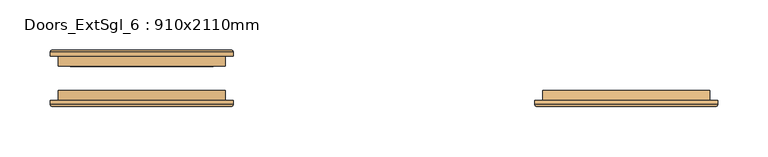
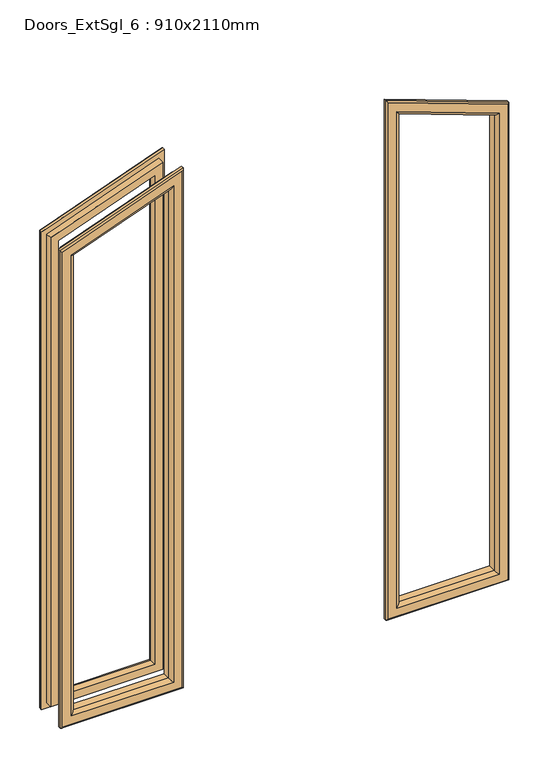
"""IFC4 building model written with IfcOpenShell, lengths in millimetres: door geometry, Doors_ExtSgl_6 : 910x2110mm."""

from ifc_helpers import new_model, si_unit, frame, origin, place, context, project, spatial, ellipse_curve, source, transform, mapped, element, save
from ifc_brep_helpers import plane_surface, cylinder_surface, advanced_brep


def doors_extsgl_6_910x2110mm_16d7c084(model_context):
    return source(origin(), model_context, "Body", "AdvancedBrep", [
        advanced_brep(
        [(323.5333333, -2.4, 1790.7556292), (323.5333333, -12.4, 1790.7556292), (323.5333333, -12.4, 1058.5), (323.5333333, -2.4, 1058.5), (311.5333333, -13.4, 1782.3531388), (311.5333333, -2.4, 1782.3531388), (311.5333333, -2.4, 1070.5), (311.5333333, -13.4, 1070.5), (316.5333333, -18.4, 1785.8541764), (316.5333333, -18.4, 1065.5), (331.5333333, -16.4, 1796.3572895), (329.5333333, -18.4, 1794.9568744), (329.5333333, -18.4, 1052.5), (331.5333333, -16.4, 1050.5), (331.5333333, -12.4, 1796.3572895), (331.5333333, -12.4, 1050.5), (157.8666667, -12.4, 1058.5), (157.8666667, -2.4, 1058.5), (169.8666667, -2.4, 1070.5), (169.8666667, -13.4, 1070.5), (164.8666667, -18.4, 1065.5), (151.8666667, -18.4, 1052.5), (149.8666667, -16.4, 1050.5), (149.8666667, -12.4, 1050.5), (157.8666667, -12.4, 1851.0533647), (157.8666667, -2.4, 1851.0533647), (169.8666667, -2.4, 1833.9155886), (169.8666667, -13.4, 1833.9155886), (164.8666667, -18.4, 1841.0563286), (151.8666667, -18.4, 1859.6222527), (149.8666667, -16.4, 1862.4785487), (149.8666667, -12.4, 1862.4785487)],
        [
            (0, 1),
            (1, 2),
            (2, 3),
            (3, 0),
            (4, 5),
            (5, 6),
            (6, 7),
            (7, 4),
            (8, 4, ellipse_curve(frame((316.5333333, -13.4, 1785.8541764), z_axis=(0.5735764363510455, 0.0, -0.8191520442889922), x_axis=(0.8191520442889922, 0.0, 0.5735764363510455)), 6.1038729, 5.0)),
            (7, 9, ellipse_curve(frame((316.5333333, -13.4, 1065.5), z_axis=(0.7071067811865475, 0.0, 0.7071067811865475), x_axis=(-0.7071067811865474, 0.0, 0.7071067811865476)), 7.0710678, 5.0)),
            (9, 8),
            (10, 11, ellipse_curve(frame((329.5333333, -16.4, 1794.9568744), z_axis=(0.5735764363510455, 0.0, -0.8191520442889922), x_axis=(0.8191520442889922, 0.0, 0.5735764363510455)), 2.4415492, 2.0)),
            (11, 12),
            (12, 13, ellipse_curve(frame((329.5333333, -16.4, 1052.5), z_axis=(0.7071067811865475, 0.0, 0.7071067811865475), x_axis=(-0.7071067811865474, 0.0, 0.7071067811865476)), 2.8284271, 2.0)),
            (13, 10),
            (14, 10),
            (13, 15),
            (15, 14),
            (2, 16),
            (16, 17),
            (17, 3),
            (6, 18),
            (18, 19),
            (19, 7),
            (19, 20, ellipse_curve(frame((164.8666667, -13.4, 1065.5), z_axis=(0.7071067811865475, 0.0, -0.7071067811865475), x_axis=(0.7071067811865476, 0.0, 0.7071067811865474)), 7.0710678, 5.0)),
            (20, 9),
            (12, 21),
            (21, 22, ellipse_curve(frame((151.8666667, -16.4, 1052.5), z_axis=(0.7071067811865475, 0.0, -0.7071067811865475), x_axis=(0.7071067811865476, 0.0, 0.7071067811865474)), 2.8284271, 2.0)),
            (22, 13),
            (22, 23),
            (23, 15),
            (16, 24),
            (24, 25),
            (25, 17),
            (18, 26),
            (26, 27),
            (27, 19),
            (27, 28, ellipse_curve(frame((164.8666667, -13.4, 1841.0563286), z_axis=(-0.8191520442889922, 0.0, -0.5735764363510455), x_axis=(0.5735764363510455, 0.0, -0.8191520442889922)), 8.717234, 5.0)),
            (28, 20),
            (21, 29),
            (29, 30, ellipse_curve(frame((151.8666667, -16.4, 1859.6222527), z_axis=(-0.8191520442889922, 0.0, -0.5735764363510455), x_axis=(0.5735764363510455, 0.0, -0.8191520442889922)), 3.4868936, 2.0)),
            (30, 22),
            (30, 31),
            (31, 23),
            (31, 14),
            (1, 24),
            (0, 25),
            (5, 26),
            (4, 27),
            (8, 28),
            (11, 29),
            (10, 30),
        ],
        [
            plane_surface(frame((323.5333333, -12.4, 1790.7556292), z_axis=(1.0, 0.0, 0.0), x_axis=(0.0, 0.0, -1.0))),
            plane_surface(frame((311.5333333, -2.4, 1782.3531388), z_axis=(-1.0, 0.0, 0.0), x_axis=(0.0, 0.0, -1.0))),
            cylinder_surface(frame((316.5333333, -13.4, 1790.7556292), z_axis=(0.0, 0.0, 1.0), x_axis=(1.0, 0.0, 0.0)), 5.0),
            cylinder_surface(frame((329.5333333, -16.4, 1790.7556292), z_axis=(0.0, 0.0, 1.0), x_axis=(1.0, 0.0, 0.0)), 2.0),
            plane_surface(frame((331.5333333, -16.4, 1796.3572895), z_axis=(1.0, 0.0, 0.0), x_axis=(0.0, 0.0, -1.0))),
            plane_surface(frame((323.5333333, -12.4, 1058.5), z_axis=(0.0, 0.0, -1.0), x_axis=(-1.0, 0.0, 0.0))),
            plane_surface(frame((311.5333333, -2.4, 1070.5), z_axis=(0.0, 0.0, 1.0), x_axis=(-1.0, 0.0, 0.0))),
            cylinder_surface(frame((323.5333333, -13.4, 1065.5), z_axis=(1.0, 0.0, 0.0), x_axis=(0.0, 0.0, -1.0)), 5.0),
            cylinder_surface(frame((323.5333333, -16.4, 1052.5), z_axis=(1.0, 0.0, 0.0), x_axis=(0.0, 0.0, -1.0)), 2.0),
            plane_surface(frame((331.5333333, -16.4, 1050.5), z_axis=(0.0, 0.0, -1.0), x_axis=(-1.0, 0.0, 0.0))),
            plane_surface(frame((157.8666667, -12.4, 1058.5), z_axis=(-1.0, 0.0, 0.0), x_axis=(0.0, 0.0, 1.0))),
            plane_surface(frame((169.8666667, -2.4, 1070.5), z_axis=(1.0, 0.0, 0.0), x_axis=(0.0, 0.0, 1.0))),
            cylinder_surface(frame((164.8666667, -13.4, 1058.5), z_axis=(0.0, 0.0, -1.0), x_axis=(-1.0, 0.0, 0.0)), 5.0),
            cylinder_surface(frame((151.8666667, -16.4, 1058.5), z_axis=(0.0, 0.0, -1.0), x_axis=(-1.0, 0.0, 0.0)), 2.0),
            plane_surface(frame((149.8666667, -16.4, 1050.5), z_axis=(-1.0, 0.0, 0.0), x_axis=(0.0, 0.0, 1.0))),
            plane_surface(frame((149.8666667, -12.4, 1862.4785487), z_axis=(0.0, 1.0000000000000002, 0.0), x_axis=(0.9396926207859077, 0.0, -0.342020143325671))),
            plane_surface(frame((157.8666667, -12.4, 1851.0533647), z_axis=(0.34202014332567127, 0.0, 0.9396926207859075), x_axis=(0.9396926207859075, 0.0, -0.34202014332567127))),
            plane_surface(frame((157.8666667, -2.4, 1851.0533647), z_axis=(0.0, 1.0, 0.0), x_axis=(0.9396926207859079, 0.0, -0.3420201433256702))),
            plane_surface(frame((169.8666667, -2.4, 1833.9155886), z_axis=(-0.34202014332566966, 0.0, -0.9396926207859081), x_axis=(0.9396926207859081, 0.0, -0.34202014332566966))),
            cylinder_surface(frame((155.4725257, -13.4, 1844.4755163), z_axis=(-0.9396926207859079, 0.0, 0.3420201433256702), x_axis=(0.3420201433256702, 0.0, 0.9396926207859079)), 5.0),
            plane_surface(frame((164.8666667, -18.4, 1841.0563286), z_axis=(0.0, -1.0, 0.0), x_axis=(0.9396926207859081, 0.0, -0.34202014332566943))),
            cylinder_surface(frame((159.9187875, -16.4, 1856.6915204), z_axis=(-0.9396926207859079, 0.0, 0.3420201433256702), x_axis=(0.3420201433256702, 0.0, 0.9396926207859079)), 2.0),
            plane_surface(frame((149.8666667, -16.4, 1862.4785487), z_axis=(0.3420201433256701, 0.0, 0.9396926207859079), x_axis=(0.9396926207859079, 0.0, -0.3420201433256701))),
        ],
        [
            (0, [[1, 2, 3, 4]]),
            (1, [[5, 6, 7, 8]]),
            (2, [[9, -8, 10, 11]]),
            (3, [[12, 13, 14, 15]]),
            (4, [[16, -15, 17, 18]]),
            (5, [[-3, 19, 20, 21]]),
            (6, [[-7, 22, 23, 24]]),
            (7, [[-10, -24, 25, 26]]),
            (8, [[-14, 27, 28, 29]]),
            (9, [[-17, -29, 30, 31]]),
            (10, [[-20, 32, 33, 34]]),
            (11, [[-23, 35, 36, 37]]),
            (12, [[-25, -37, 38, 39]]),
            (13, [[-28, 40, 41, 42]]),
            (14, [[-30, -42, 43, 44]]),
            (15, [[-31, -44, 45, -18], [46, -32, -19, -2]]),
            (16, [[-33, -46, -1, 47]]),
            (17, [[-21, -34, -47, -4], [48, -35, -22, -6]]),
            (18, [[-36, -48, -5, 49]]),
            (19, [[-38, -49, -9, 50]]),
            (20, [[51, -40, -27, -13], [-26, -39, -50, -11]]),
            (21, [[-41, -51, -12, 52]]),
            (22, [[-43, -52, -16, -45]]),
        ],
    ),
        advanced_brep(
        [(-149.8, 35.6, 1050.5), (-149.8, 31.6, 1050.5), (-331.4666667, 31.6, 1050.5), (-331.4666667, 35.6, 1050.5), (-151.8, 37.6, 1052.5), (-329.4666667, 37.6, 1052.5), (-169.8, 32.6, 1070.5), (-164.8, 37.6, 1065.5), (-316.4666667, 37.6, 1065.5), (-311.4666667, 32.6, 1070.5), (-169.8, 21.6, 1070.5), (-311.4666667, 21.6, 1070.5), (-157.8, 31.6, 1058.5), (-157.8, 21.6, 1058.5), (-323.4666667, 21.6, 1058.5), (-323.4666667, 31.6, 1058.5), (-331.4666667, 31.6, 1796.3572895), (-331.4666667, 35.6, 1796.3572895), (-329.4666667, 37.6, 1794.9568744), (-316.4666667, 37.6, 1785.8541764), (-311.4666667, 32.6, 1782.3531388), (-311.4666667, 21.6, 1782.3531388), (-323.4666667, 21.6, 1790.7556292), (-323.4666667, 31.6, 1790.7556292), (-149.8, 31.6, 1862.4785487), (-149.8, 35.6, 1862.4785487), (-151.8, 37.6, 1859.6222527), (-164.8, 37.6, 1841.0563286), (-169.8, 32.6, 1833.9155886), (-169.8, 21.6, 1833.9155886), (-157.8, 21.6, 1851.0533647), (-157.8, 31.6, 1851.0533647)],
        [
            (0, 1),
            (1, 2),
            (2, 3),
            (3, 0),
            (4, 0, ellipse_curve(frame((-151.8, 35.6, 1052.5), z_axis=(-0.7071067811865476, 0.0, -0.7071067811865475), x_axis=(0.7071067811865474, 0.0, -0.7071067811865476)), 2.8284271, 2.0)),
            (3, 5, ellipse_curve(frame((-329.4666667, 35.6, 1052.5), z_axis=(0.7071067811865475, 0.0, -0.7071067811865476), x_axis=(0.7071067811865476, 0.0, 0.7071067811865474)), 2.8284271, 2.0)),
            (5, 4),
            (6, 7, ellipse_curve(frame((-164.8, 32.6, 1065.5), z_axis=(-0.7071067811865476, 0.0, -0.7071067811865475), x_axis=(0.7071067811865474, 0.0, -0.7071067811865476)), 7.0710678, 5.0)),
            (7, 8),
            (8, 9, ellipse_curve(frame((-316.4666667, 32.6, 1065.5), z_axis=(0.7071067811865475, 0.0, -0.7071067811865476), x_axis=(0.7071067811865476, 0.0, 0.7071067811865474)), 7.0710678, 5.0)),
            (9, 6),
            (10, 6),
            (9, 11),
            (11, 10),
            (12, 13),
            (13, 14),
            (14, 15),
            (15, 12),
            (2, 16),
            (16, 17),
            (17, 3),
            (17, 18, ellipse_curve(frame((-329.4666667, 35.6, 1794.9568744), z_axis=(-0.5735764363510453, 0.0, -0.8191520442889924), x_axis=(0.8191520442889924, 0.0, -0.5735764363510454)), 2.4415492, 2.0)),
            (18, 5),
            (8, 19),
            (19, 20, ellipse_curve(frame((-316.4666667, 32.6, 1785.8541764), z_axis=(-0.5735764363510453, 0.0, -0.8191520442889924), x_axis=(0.8191520442889924, 0.0, -0.5735764363510454)), 6.1038729, 5.0)),
            (20, 9),
            (20, 21),
            (21, 11),
            (14, 22),
            (22, 23),
            (23, 15),
            (16, 24),
            (24, 25),
            (25, 17),
            (25, 26, ellipse_curve(frame((-151.8, 35.6, 1859.6222527), z_axis=(-0.8191520442889924, 0.0, 0.5735764363510453), x_axis=(-0.5735764363510453, 0.0, -0.8191520442889924)), 3.4868936, 2.0)),
            (26, 18),
            (19, 27),
            (27, 28, ellipse_curve(frame((-164.8, 32.6, 1841.0563286), z_axis=(-0.8191520442889924, 0.0, 0.5735764363510453), x_axis=(-0.5735764363510453, 0.0, -0.8191520442889924)), 8.717234, 5.0)),
            (28, 20),
            (28, 29),
            (29, 21),
            (22, 30),
            (30, 31),
            (31, 23),
            (24, 1),
            (0, 25),
            (4, 26),
            (7, 27),
            (6, 28),
            (10, 29),
            (13, 30),
            (12, 31),
        ],
        [
            plane_surface(frame((-149.8, 31.6, 1050.5), z_axis=(0.0, 0.0, -1.0), x_axis=(-1.0, 0.0, 0.0))),
            cylinder_surface(frame((-157.8, 35.6, 1052.5), z_axis=(1.0, 0.0, 0.0), x_axis=(0.0, 0.0, -1.0)), 2.0),
            cylinder_surface(frame((-157.8, 32.6, 1065.5), z_axis=(1.0, 0.0, 0.0), x_axis=(0.0, 0.0, -1.0)), 5.0),
            plane_surface(frame((-169.8, 32.6, 1070.5), z_axis=(0.0, 0.0, 1.0), x_axis=(-1.0, 0.0, 0.0))),
            plane_surface(frame((-157.8, 21.6, 1058.5), z_axis=(0.0, 0.0, -1.0), x_axis=(-1.0, 0.0, 0.0))),
            plane_surface(frame((-331.4666667, 31.6, 1050.5), z_axis=(-1.0, 0.0, 0.0), x_axis=(0.0, 0.0, 1.0))),
            cylinder_surface(frame((-329.4666667, 35.6, 1058.5), z_axis=(0.0, 0.0, -1.0), x_axis=(-1.0, 0.0, 0.0)), 2.0),
            cylinder_surface(frame((-316.4666667, 32.6, 1058.5), z_axis=(0.0, 0.0, -1.0), x_axis=(-1.0, 0.0, 0.0)), 5.0),
            plane_surface(frame((-311.4666667, 32.6, 1070.5), z_axis=(1.0, 0.0, 0.0), x_axis=(0.0, 0.0, 1.0))),
            plane_surface(frame((-323.4666667, 21.6, 1058.5), z_axis=(-1.0, 0.0, 0.0), x_axis=(0.0, 0.0, 1.0))),
            plane_surface(frame((-331.4666667, 31.6, 1796.3572895), z_axis=(-0.34202014332567054, 0.0, 0.9396926207859078), x_axis=(0.9396926207859078, 0.0, 0.34202014332567054))),
            cylinder_surface(frame((-325.5187875, 35.6, 1796.3937849), z_axis=(-0.9396926207859077, 0.0, -0.34202014332567077), x_axis=(-0.34202014332567077, 0.0, 0.9396926207859077)), 2.0),
            cylinder_surface(frame((-321.0725257, 32.6, 1784.1777809), z_axis=(-0.9396926207859077, 0.0, -0.34202014332567077), x_axis=(-0.34202014332567077, 0.0, 0.9396926207859077)), 5.0),
            plane_surface(frame((-311.4666667, 32.6, 1782.3531388), z_axis=(0.34202014332567, 0.0, -0.939692620785908), x_axis=(0.939692620785908, 0.0, 0.34202014332567))),
            plane_surface(frame((-323.4666667, 21.6, 1790.7556292), z_axis=(-0.3420201433256708, 0.0, 0.9396926207859077), x_axis=(0.9396926207859077, 0.0, 0.3420201433256708))),
            plane_surface(frame((-149.8, 31.6, 1862.4785487), z_axis=(1.0, 0.0, 0.0), x_axis=(0.0, 0.0, -1.0))),
            cylinder_surface(frame((-151.8, 35.6, 1851.0533647), z_axis=(0.0, 0.0, 1.0), x_axis=(1.0, 0.0, 0.0)), 2.0),
            plane_surface(frame((-151.8, 37.6, 1859.6222527), z_axis=(0.0, 1.0, 0.0), x_axis=(0.0, 0.0, -1.0))),
            cylinder_surface(frame((-164.8, 32.6, 1851.0533647), z_axis=(0.0, 0.0, 1.0), x_axis=(1.0, 0.0, 0.0)), 5.0),
            plane_surface(frame((-169.8, 32.6, 1833.9155886), z_axis=(-1.0, 0.0, 0.0), x_axis=(0.0, 0.0, -1.0))),
            plane_surface(frame((-169.8, 21.6, 1833.9155886), z_axis=(0.0, -1.0, 0.0), x_axis=(0.0, 0.0, -1.0))),
            plane_surface(frame((-157.8, 21.6, 1851.0533647), z_axis=(1.0, 0.0, 0.0), x_axis=(0.0, 0.0, -1.0))),
            plane_surface(frame((-157.8, 31.6, 1851.0533647), z_axis=(0.0, -1.0, 0.0), x_axis=(0.0, 0.0, -1.0))),
        ],
        [
            (0, [[1, 2, 3, 4]]),
            (1, [[5, -4, 6, 7]]),
            (2, [[8, 9, 10, 11]]),
            (3, [[12, -11, 13, 14]]),
            (4, [[15, 16, 17, 18]]),
            (5, [[-3, 19, 20, 21]]),
            (6, [[-6, -21, 22, 23]]),
            (7, [[-10, 24, 25, 26]]),
            (8, [[-13, -26, 27, 28]]),
            (9, [[-17, 29, 30, 31]]),
            (10, [[-20, 32, 33, 34]]),
            (11, [[-22, -34, 35, 36]]),
            (12, [[-25, 37, 38, 39]]),
            (13, [[-27, -39, 40, 41]]),
            (14, [[-30, 42, 43, 44]]),
            (15, [[-33, 45, -1, 46]]),
            (16, [[-35, -46, -5, 47]]),
            (17, [[-23, -36, -47, -7], [48, -37, -24, -9]]),
            (18, [[-38, -48, -8, 49]]),
            (19, [[-40, -49, -12, 50]]),
            (20, [[51, -42, -29, -16], [-28, -41, -50, -14]]),
            (21, [[-43, -51, -15, 52]]),
            (22, [[-45, -32, -19, -2], [-31, -44, -52, -18]]),
        ],
    ),
        advanced_brep(
        [(-323.4666667, -2.4, 1790.7556292), (-323.4666667, -12.4, 1790.7556292), (-157.8, -12.4, 1851.0533647), (-157.8, -2.4, 1851.0533647), (-311.4666667, -13.4, 1782.3531388), (-311.4666667, -2.4, 1782.3531388), (-169.8, -2.4, 1833.9155886), (-169.8, -13.4, 1833.9155886), (-316.4666667, -18.4, 1785.8541764), (-164.8, -18.4, 1841.0563286), (-331.4666667, -16.4, 1796.3572895), (-329.4666667, -18.4, 1794.9568744), (-151.8, -18.4, 1859.6222527), (-149.8, -16.4, 1862.4785487), (-331.4666667, -12.4, 1796.3572895), (-149.8, -12.4, 1862.4785487), (-157.8, -12.4, 1058.5), (-157.8, -2.4, 1058.5), (-169.8, -2.4, 1070.5), (-169.8, -13.4, 1070.5), (-164.8, -18.4, 1065.5), (-151.8, -18.4, 1052.5), (-149.8, -16.4, 1050.5), (-149.8, -12.4, 1050.5), (-323.4666667, -12.4, 1058.5), (-323.4666667, -2.4, 1058.5), (-311.4666667, -2.4, 1070.5), (-311.4666667, -13.4, 1070.5), (-316.4666667, -18.4, 1065.5), (-329.4666667, -18.4, 1052.5), (-331.4666667, -16.4, 1050.5), (-331.4666667, -12.4, 1050.5)],
        [
            (0, 1),
            (1, 2),
            (2, 3),
            (3, 0),
            (4, 5),
            (5, 6),
            (6, 7),
            (7, 4),
            (8, 4, ellipse_curve(frame((-316.4666667, -13.4, 1785.8541764), z_axis=(0.5735764363510448, 0.0, 0.8191520442889929), x_axis=(-0.8191520442889925, 0.0, 0.5735764363510449)), 6.1038729, 5.0)),
            (7, 9, ellipse_curve(frame((-164.8, -13.4, 1841.0563286), z_axis=(-0.8191520442889928, 0.0, 0.5735764363510447), x_axis=(-0.5735764363510447, 0.0, -0.8191520442889929)), 8.717234, 5.0)),
            (9, 8),
            (10, 11, ellipse_curve(frame((-329.4666667, -16.4, 1794.9568744), z_axis=(0.5735764363510448, 0.0, 0.8191520442889929), x_axis=(-0.8191520442889925, 0.0, 0.5735764363510449)), 2.4415492, 2.0)),
            (11, 12),
            (12, 13, ellipse_curve(frame((-151.8, -16.4, 1859.6222527), z_axis=(-0.8191520442889928, 0.0, 0.5735764363510447), x_axis=(-0.5735764363510447, 0.0, -0.8191520442889929)), 3.4868936, 2.0)),
            (13, 10),
            (14, 10),
            (13, 15),
            (15, 14),
            (2, 16),
            (16, 17),
            (17, 3),
            (6, 18),
            (18, 19),
            (19, 7),
            (19, 20, ellipse_curve(frame((-164.8, -13.4, 1065.5), z_axis=(0.7071067811865471, 0.0, 0.7071067811865479), x_axis=(-0.7071067811865479, 0.0, 0.707106781186547)), 7.0710678, 5.0)),
            (20, 9),
            (12, 21),
            (21, 22, ellipse_curve(frame((-151.8, -16.4, 1052.5), z_axis=(0.7071067811865471, 0.0, 0.7071067811865479), x_axis=(-0.7071067811865479, 0.0, 0.707106781186547)), 2.8284271, 2.0)),
            (22, 13),
            (22, 23),
            (23, 15),
            (16, 24),
            (24, 25),
            (25, 17),
            (18, 26),
            (26, 27),
            (27, 19),
            (27, 28, ellipse_curve(frame((-316.4666667, -13.4, 1065.5), z_axis=(0.7071067811865478, 0.0, -0.7071067811865471), x_axis=(0.7071067811865474, 0.0, 0.7071067811865476)), 7.0710678, 5.0)),
            (28, 20),
            (21, 29),
            (29, 30, ellipse_curve(frame((-329.4666667, -16.4, 1052.5), z_axis=(0.7071067811865478, 0.0, -0.7071067811865471), x_axis=(0.7071067811865474, 0.0, 0.7071067811865476)), 2.8284271, 2.0)),
            (30, 22),
            (30, 31),
            (31, 23),
            (31, 14),
            (1, 24),
            (0, 25),
            (5, 26),
            (4, 27),
            (8, 28),
            (11, 29),
            (10, 30),
        ],
        [
            plane_surface(frame((-323.4666667, -12.4, 1790.7556292), z_axis=(-0.3420201433256702, 0.0, 0.9396926207859079), x_axis=(0.9396926207859079, 0.0, 0.3420201433256702))),
            plane_surface(frame((-311.4666667, -2.4, 1782.3531388), z_axis=(0.3420201433256704, 0.0, -0.9396926207859078), x_axis=(0.9396926207859078, 0.0, 0.3420201433256704))),
            cylinder_surface(frame((-321.0725257, -13.4, 1784.1777809), z_axis=(-0.9396926207859074, 0.0, -0.34202014332567143), x_axis=(-0.34202014332567143, 0.0, 0.9396926207859074)), 5.0),
            cylinder_surface(frame((-325.5187875, -16.4, 1796.3937849), z_axis=(-0.9396926207859074, 0.0, -0.34202014332567143), x_axis=(-0.34202014332567143, 0.0, 0.9396926207859074)), 2.0),
            plane_surface(frame((-331.4666667, -16.4, 1796.3572895), z_axis=(-0.34202014332567077, 0.0, 0.9396926207859077), x_axis=(0.9396926207859077, 0.0, 0.34202014332567077))),
            plane_surface(frame((-157.8, -12.4, 1851.0533647), z_axis=(1.0, 0.0, 0.0), x_axis=(0.0, 0.0, -1.0))),
            plane_surface(frame((-169.8, -2.4, 1833.9155886), z_axis=(-1.0, 0.0, 0.0), x_axis=(0.0, 0.0, -1.0))),
            cylinder_surface(frame((-164.8, -13.4, 1851.0533647), z_axis=(0.0, 0.0, 1.0), x_axis=(1.0, 0.0, 0.0)), 5.0),
            cylinder_surface(frame((-151.8, -16.4, 1851.0533647), z_axis=(0.0, 0.0, 1.0), x_axis=(1.0, 0.0, 0.0)), 2.0),
            plane_surface(frame((-149.8, -16.4, 1862.4785487), z_axis=(1.0, 0.0, 0.0), x_axis=(0.0, 0.0, -1.0))),
            plane_surface(frame((-157.8, -12.4, 1058.5), z_axis=(0.0, 0.0, -1.0), x_axis=(-1.0, 0.0, 0.0))),
            plane_surface(frame((-169.8, -2.4, 1070.5), z_axis=(0.0, 0.0, 1.0), x_axis=(-1.0, 0.0, 0.0))),
            cylinder_surface(frame((-157.8, -13.4, 1065.5), z_axis=(1.0, 0.0, 0.0), x_axis=(0.0, 0.0, -1.0)), 5.0),
            cylinder_surface(frame((-157.8, -16.4, 1052.5), z_axis=(1.0, 0.0, 0.0), x_axis=(0.0, 0.0, -1.0)), 2.0),
            plane_surface(frame((-149.8, -16.4, 1050.5), z_axis=(0.0, 0.0, -1.0), x_axis=(-1.0, 0.0, 0.0))),
            plane_surface(frame((-331.4666667, -12.4, 1050.5), z_axis=(0.0, 1.0, 0.0), x_axis=(0.0, 0.0, 1.0))),
            plane_surface(frame((-323.4666667, -12.4, 1058.5), z_axis=(-1.0, 0.0, 0.0), x_axis=(0.0, 0.0, 1.0))),
            plane_surface(frame((-323.4666667, -2.4, 1058.5), z_axis=(0.0, 1.0, 0.0), x_axis=(0.0, 0.0, 1.0))),
            plane_surface(frame((-311.4666667, -2.4, 1070.5), z_axis=(1.0, 0.0, 0.0), x_axis=(0.0, 0.0, 1.0))),
            cylinder_surface(frame((-316.4666667, -13.4, 1058.5), z_axis=(0.0, 0.0, -1.0), x_axis=(-1.0, 0.0, 0.0)), 5.0),
            plane_surface(frame((-316.4666667, -18.4, 1065.5), z_axis=(0.0, -1.0, 0.0), x_axis=(0.0, 0.0, 1.0))),
            cylinder_surface(frame((-329.4666667, -16.4, 1058.5), z_axis=(0.0, 0.0, -1.0), x_axis=(-1.0, 0.0, 0.0)), 2.0),
            plane_surface(frame((-331.4666667, -16.4, 1050.5), z_axis=(-1.0, 0.0, 0.0), x_axis=(0.0, 0.0, 1.0))),
        ],
        [
            (0, [[1, 2, 3, 4]]),
            (1, [[5, 6, 7, 8]]),
            (2, [[9, -8, 10, 11]]),
            (3, [[12, 13, 14, 15]]),
            (4, [[16, -15, 17, 18]]),
            (5, [[-3, 19, 20, 21]]),
            (6, [[-7, 22, 23, 24]]),
            (7, [[-10, -24, 25, 26]]),
            (8, [[-14, 27, 28, 29]]),
            (9, [[-17, -29, 30, 31]]),
            (10, [[-20, 32, 33, 34]]),
            (11, [[-23, 35, 36, 37]]),
            (12, [[-25, -37, 38, 39]]),
            (13, [[-28, 40, 41, 42]]),
            (14, [[-30, -42, 43, 44]]),
            (15, [[-31, -44, 45, -18], [46, -32, -19, -2]]),
            (16, [[-33, -46, -1, 47]]),
            (17, [[-21, -34, -47, -4], [48, -35, -22, -6]]),
            (18, [[-36, -48, -5, 49]]),
            (19, [[-38, -49, -9, 50]]),
            (20, [[51, -40, -27, -13], [-26, -39, -50, -11]]),
            (21, [[-41, -51, -12, 52]]),
            (22, [[-43, -52, -16, -45]]),
        ],
    ),
    ])


if __name__ == "__main__":
    model = new_model("IFC4")
    model_context = context("Model", 3, world=origin())
    ifc_project = project(units=[si_unit("LENGTHUNIT", "METRE", prefix="MILLI")], contexts=[model_context])
    site = spatial("IfcSite", under=ifc_project)
    building = spatial("IfcBuilding", under=site)
    placement = place(None, origin())
    doors_extsgl_6_910x2110mm_shape = doors_extsgl_6_910x2110mm_16d7c084(model_context)
    element("IfcDoor", 1, ObjectType="Doors_ExtSgl_6 : 910x2110mm", at=placement, inside=building, context=model_context, shape_type="MappedRepresentation", body=[
        mapped(doors_extsgl_6_910x2110mm_shape, transform((0.0, 0.0, 0.0), x_axis=(1.0, 0.0, 0.0), y_axis=(0.0, 1.0, 0.0), z_axis=(0.0, 0.0, 1.0))),
    ])
    save(model, "model.ifc")

# Revit data of these elements
# Type "Doors_ExtSgl_6 : 910x2110mm"
#   Type Mark = "13"
#   Type Comments = "External Single"
#   Operation = "SingleSwingRight"
#   Construction Type Id = "SGL"
#   Keynote = "L20"
#   Analytic Construction = "Large single-glazed windows"
#   Wrap Layers (Int) from Ext = 0' - 6.98819"
#   Wrap Layers (Ext) from Ext = 0' - 4.03543"
#   Visual Light Transmittance = 0.9
#   Thickness = 0' - 1.73228"
#   Stile Top of Lock rail = 3' - 3.37008"
#   Stile Top Rail = 0' - 5.90551"
#   Stile Shutting = 0' - 3.14961"
#   Stile Muntin Rail = 0' - 2.95276"
#   Stile Lock Rail = 0' - 6.88976"
#   Stile Hanging = 0' - 3.14961"
#   Stile Bottom Rail = 0' - 6.88976"
#   Solar Heat Gain Coefficient = 0.86
#   Rough Width = 2' - 11.82677"
#   Rough Height = 6' - 11.07087"
#   O/A Frame Width = 0' - 2.51969"
#   Heat Transfer Coefficient (U) = 0.979472 BTU/(h·ft²·°F)
#   Handle Z Distance = 3' - 3.37008"
#   Glazing Thickness = 0' - 0.94488"
#   FrameWidth = 0' - 1.65354"
#   FrameOffset - External = 0' - 0.98425"
#   FrameDepth = 0' - 3.50394"
#   Door Panel Width = 2' - 7.77165"
#   Door Panel Thickness = 0' - 1.73228"
#   Door Panel Height = 6' - 6.74016"
#   DONT CHANGE - Panel Width = 0' - 6.52231"
#   Cill Thickness = 0' - 2.14567"
#   Cill Projection = 0' - 1.1811"
#   Handle X Distance = 0' - 2.95276"
#   Height = 6' - 11.07087"
#   Structural Tolerance = 0' - 0.25591"
#   Tolerance = 0' - 0.11811"
#   Undercut = 0' - 0.15748"
#   Width = 2' - 11.82677"
#   Cill Extension = 0' - 0.98425"
#   Cavity Closer Width = 0' - 1.9685"
#   Cavity Closer Offset from Ext = 0' - 4.03543"
#   Cavity Closer Depth = 0' - 3.34646"
#   Vis - Ironmongery = yes
#   Vis - Cavity Closers = yes
#   Define Thermal Properties by = 1
#   Function = 1
#   Material Glass = Door - Glazing
#   Material Door = Door - Panel
#   Material Frame = Door - Frame/Mullion
#   Material Ironmongery = Door - Handle
#   Wall Closure = (empty or 0)
# Element 1 (IfcDoor, "Doors_ExtSgl_6 : 910x2110mm")
#   Materials on its faces: "Door - Panel", "Door - Handle", "Door - Frame/Mullion", "Door - Glazing"
# Materials
#   "Door - Glazing": colour RGB 0 0 255, transparency 0.75
#   "Door - Panel": class "Wood", colour RGB 210 159 95, transparency 0, Cost = 0
#   "Door - Frame/Mullion": class "Wood", colour RGB 212 179 113, transparency 0
#   "Door - Handle": colour RGB 0 0 0, transparency 0
